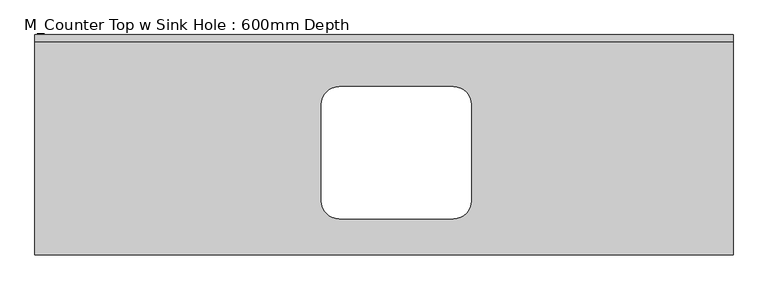
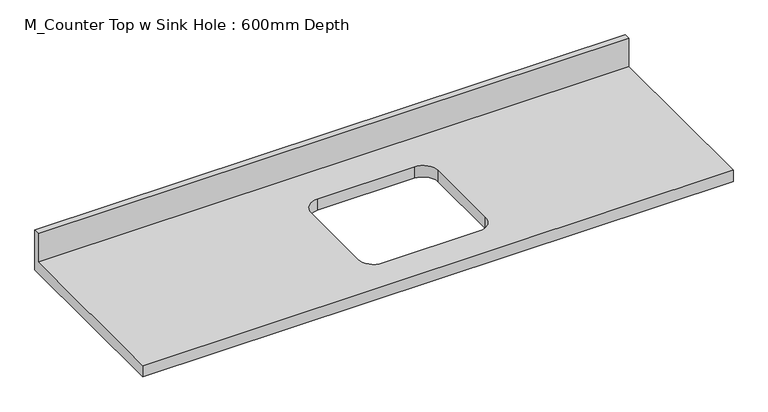
"""IFC4 building model written with IfcOpenShell, lengths in millimetres: furniture geometry, M_Counter Top w Sink Hole : 600mm Depth."""

from ifc_helpers import new_model, si_unit, frame, origin, place, context, project, spatial, polyline, circle_curve, source, transform, mapped, element, save
from ifc_brep_helpers import plane_surface, revolved_surface, advanced_brep


def m_counter_top_w_sink_hole_600mm_depth_0a237b63(model_context):
    return source(origin(), model_context, "Body", "AdvancedBrep", [
        advanced_brep(
        [(-1200.4622951, -625.0, 900.0), (779.5377049, -625.0, 900.0), (779.5377049, -19.05, 900.0), (-1200.4622951, -19.05, 900.0), (-337.3622951, -147.3, 900.0), (-13.5622951, -147.3, 900.0), (37.2377049, -198.1, 900.0), (37.2377049, -471.9, 900.0), (-13.5622951, -522.7, 900.0), (-337.3622951, -522.7, 900.0), (-388.1622951, -471.9, 900.0), (-388.1622951, -198.1, 900.0), (779.5377049, 0.0, 860.0), (779.5377049, -625.0, 860.0), (-1200.4622951, -625.0, 860.0), (-1200.4622951, 0.0, 860.0), (-13.5622951, -147.3, 860.0), (-337.3622951, -147.3, 860.0), (-388.1622951, -198.1, 860.0), (-388.1622951, -471.9, 860.0), (-337.3622951, -522.7, 860.0), (-13.5622951, -522.7, 860.0), (37.2377049, -471.9, 860.0), (37.2377049, -198.1, 860.0), (-1200.4622951, 0.0, 1001.6), (779.5377049, 0.0, 1001.6), (-1200.4622951, -19.05, 1001.6), (779.5377049, -19.05, 1001.6)],
        [
            (0, 1),
            (1, 2),
            (2, 3),
            (3, 0),
            (4, 5),
            (5, 6, circle_curve(frame((-13.5622951, -198.1, 900.0), z_axis=(0.0, 0.0, -1.0), x_axis=(1.0, 0.0, 0.0)), 50.8)),
            (6, 7),
            (7, 8, circle_curve(frame((-13.5622951, -471.9, 900.0), z_axis=(0.0, 0.0, -1.0), x_axis=(1.0, 0.0, 0.0)), 50.8)),
            (8, 9),
            (9, 10, circle_curve(frame((-337.3622951, -471.9, 900.0), z_axis=(0.0, 0.0, -1.0), x_axis=(1.0, 0.0, 0.0)), 50.8)),
            (10, 11),
            (11, 4, circle_curve(frame((-337.3622951, -198.1, 900.0), z_axis=(0.0, 0.0, -1.0), x_axis=(1.0, 0.0, 0.0)), 50.8)),
            (12, 13),
            (13, 14),
            (14, 15),
            (15, 12),
            (16, 17),
            (17, 18, circle_curve(frame((-337.3622951, -198.1, 860.0), z_axis=(0.0, 0.0, 1.0), x_axis=(1.0, 0.0, 0.0)), 50.8)),
            (18, 19),
            (19, 20, circle_curve(frame((-337.3622951, -471.9, 860.0), z_axis=(0.0, 0.0, 1.0), x_axis=(1.0, 0.0, 0.0)), 50.8)),
            (20, 21),
            (21, 22, circle_curve(frame((-13.5622951, -471.9, 860.0), z_axis=(0.0, 0.0, 1.0), x_axis=(1.0, 0.0, 0.0)), 50.8)),
            (22, 23),
            (23, 16, circle_curve(frame((-13.5622951, -198.1, 860.0), z_axis=(0.0, 0.0, 1.0), x_axis=(1.0, 0.0, 0.0)), 50.8)),
            (15, 24),
            (24, 25),
            (25, 12),
            (14, 0),
            (3, 26),
            (26, 24),
            (13, 1),
            (25, 27),
            (27, 2),
            (26, 27),
            (4, 17),
            (16, 5),
            (11, 18),
            (10, 19),
            (9, 20),
            (8, 21),
            (7, 22),
            (6, 23),
        ],
        [
            plane_surface(frame((-1200.4622951, 0.0, 900.0), z_axis=(0.0, 0.0, 1.0), x_axis=(-1.0, 0.0, 0.0))),
            plane_surface(frame((-1200.4622951, 0.0, 860.0), z_axis=(0.0, 0.0, -1.0), x_axis=(1.0, 0.0, 0.0))),
            plane_surface(frame((779.5377049, 0.0, 900.0), z_axis=(0.0, 1.0, 0.0), x_axis=(0.0, 0.0, -1.0))),
            plane_surface(frame((-1200.4622951, 0.0, 900.0), z_axis=(-1.0, 0.0, 0.0), x_axis=(0.0, 0.0, -1.0))),
            plane_surface(frame((-1200.4622951, -625.0, 900.0), z_axis=(0.0, -1.0, 0.0), x_axis=(0.0, 0.0, -1.0))),
            plane_surface(frame((779.5377049, -625.0, 900.0), z_axis=(1.0, 0.0, 0.0), x_axis=(0.0, 0.0, -1.0))),
            plane_surface(frame((-1200.4622951, 0.0, 1001.6), z_axis=(0.0, 0.0, 1.0), x_axis=(0.0, -1.0, 0.0))),
            plane_surface(frame((-1200.4622951, -19.05, 1001.6), z_axis=(0.0, -1.0, 0.0), x_axis=(0.0, 0.0, -1.0))),
            plane_surface(frame((-13.5622951, -147.3, 900.0), z_axis=(0.0, -1.0, 0.0), x_axis=(0.0, 0.0, -1.0))),
            revolved_surface(polyline([(-286.5622951, -198.1, 900.0), (-286.5622951, -198.1, 860.0)]), (-337.3622951, -198.1, 860.0), (0.0, 0.0, 1.0)),
            plane_surface(frame((-388.1622951, -198.1, 900.0), z_axis=(1.0, 0.0, 0.0), x_axis=(0.0, 0.0, -1.0))),
            revolved_surface(polyline([(-286.5622951, -471.9, 900.0), (-286.5622951, -471.9, 860.0)]), (-337.3622951, -471.9, 860.0), (0.0, 0.0, 1.0)),
            plane_surface(frame((-337.3622951, -522.7, 900.0), z_axis=(0.0, 1.0, 0.0), x_axis=(0.0, 0.0, -1.0))),
            revolved_surface(polyline([(37.2377049, -471.9, 900.0), (37.2377049, -471.9, 860.0)]), (-13.5622951, -471.9, 860.0), (0.0, 0.0, 1.0)),
            plane_surface(frame((37.2377049, -471.9, 900.0), z_axis=(-1.0, 0.0, 0.0), x_axis=(0.0, 0.0, -1.0))),
            revolved_surface(polyline([(37.2377049, -198.1, 900.0), (37.2377049, -198.1, 860.0)]), (-13.5622951, -198.1, 860.0), (0.0, 0.0, 1.0)),
        ],
        [
            (0, [[1, 2, 3, 4], [5, 6, 7, 8, 9, 10, 11, 12]]),
            (1, [[13, 14, 15, 16], [17, 18, 19, 20, 21, 22, 23, 24]]),
            (2, [[-16, 25, 26, 27]]),
            (3, [[-15, 28, -4, 29, 30, -25]]),
            (4, [[-1, -28, -14, 31]]),
            (5, [[-13, -27, 32, 33, -2, -31]]),
            (6, [[-30, 34, -32, -26]]),
            (7, [[-34, -29, -3, -33]]),
            (8, [[35, -17, 36, -5]]),
            (9, [[-35, -12, 37, -18]]),
            (10, [[-37, -11, 38, -19]]),
            (11, [[-38, -10, 39, -20]]),
            (12, [[-39, -9, 40, -21]]),
            (13, [[-40, -8, 41, -22]]),
            (14, [[-41, -7, 42, -23]]),
            (15, [[-36, -24, -42, -6]]),
        ],
    ),
    ])


if __name__ == "__main__":
    model = new_model("IFC4")
    model_context = context("Model", 3, world=origin())
    ifc_project = project(units=[si_unit("LENGTHUNIT", "METRE", prefix="MILLI")], contexts=[model_context])
    site = spatial("IfcSite", under=ifc_project)
    building = spatial("IfcBuilding", under=site)
    placement = place(None, origin())
    m_counter_top_w_sink_hole_600mm_depth_shape = m_counter_top_w_sink_hole_600mm_depth_0a237b63(model_context)
    element("IfcFurniture", 1, ObjectType="M_Counter Top w Sink Hole : 600mm Depth", at=placement, inside=building, context=model_context, shape_type="MappedRepresentation", body=[
        mapped(m_counter_top_w_sink_hole_600mm_depth_shape, transform((0.0, 0.0, 0.0), x_axis=(1.0, 0.0, 0.0), y_axis=(0.0, 1.0, 0.0), z_axis=(0.0, 0.0, 1.0))),
    ])
    save(model, "model.ifc")

# Revit data of these elements
# Type "M_Counter Top w Sink Hole : 600mm Depth"
#   Counter Thickness = 0' - 1.5748"
#   Depth = 2' - 0.6063"
#   Height = 2' - 11.43307"
#   Length [instance default] = 8' - 2.4252"
#   Sink Location [instance default] = 3' - 11.24409"
#   Sink Location To Wall [instance default] = 0' - 3.93701"
#   Sink Opening Depth [instance default] = 1' - 2.88189"
#   Sink Opening Width [instance default] = 1' - 11.11024"
#   Counter Top Material = none
#   Default Elevation = 0
# Element 1 (IfcFurniture, "M_Counter Top w Sink Hole : 600mm Depth")
#   Length = 6' - 5.95276"
#   Sink Location = 3' - 4.35433"
#   Sink Location To Wall = 0' - 6.29921"
#   Sink Opening Depth = 1' - 1.77953"
#   Sink Opening Width = 1' - 3.74803"
#   Materials on its faces: "Counter Top"
# Materials
#   "Counter Top": class "Wood", colour RGB 226 177 128, transparency 0
